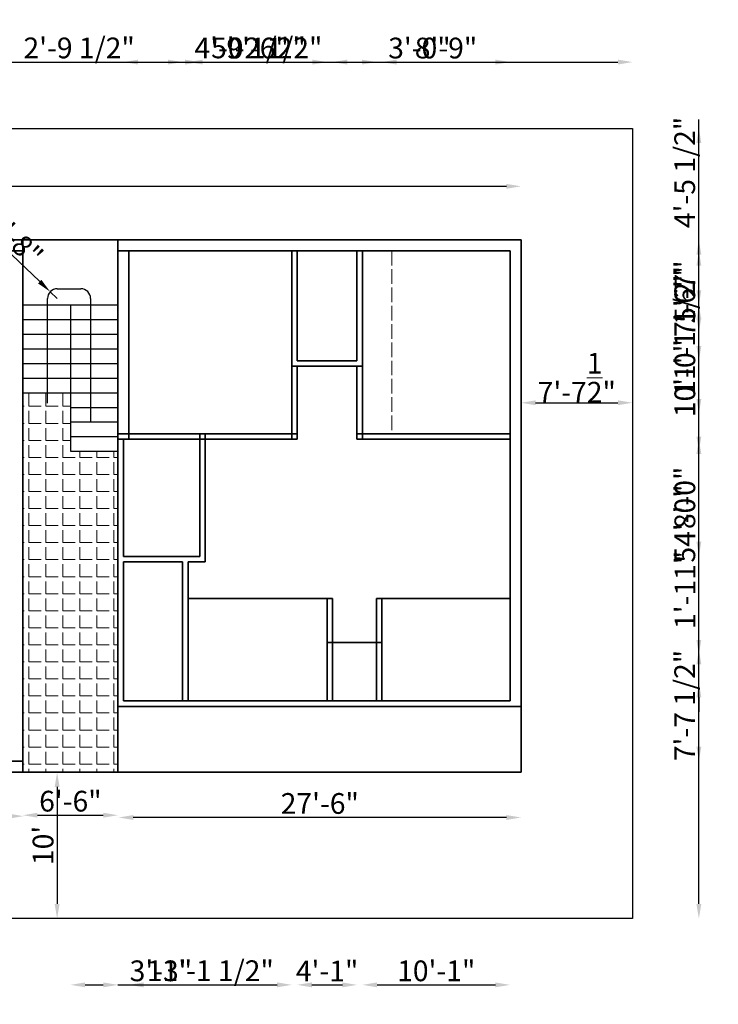
# Model space of a CAD drawing. Units: millimetres. Extents: x 1980 to 3220, y 1535 to 2343.
# Tile 3 of 3: x 2647 to 3220, y 1535 to 2343. Entities that reach past the tile are written whole.
import ezdxf

# ---------------------------------------------------------------- set-up
doc = ezdxf.new("R2010")
doc.units = ezdxf.units.MM
doc.linetypes.add('ACAD_ISO02W100', pattern=[15, 12, -3])
for name, color, linetype, lineweight in [('A-ANNO-DIMS', 2, 'Continuous', 18), ('A-FLOR-FIXT', 9, 'Continuous', 18), ('A-FLOR-FIXT-OVHD', 9, 'ACAD_ISO02W100', 18), ('A-FLOR-PATT', 252, 'Continuous', 13), ('A-FLOR-STRS', 3, 'Continuous', 25), ('A-WALL', 7, 'Continuous', 35), ('C-PROP', 8, 'Continuous', 25)]:
    doc.layers.add(name, color=color, linetype=linetype, lineweight=lineweight)
doc.styles.get("Standard").update_dxf_attribs({"font": 'arial.ttf'})
doc.dimstyles.new('ISO-25', dxfattribs={"dimtxt": 17, "dimasz": 12, "dimexe": 1.25, "dimexo": 0.625, "dimtad": 1, "dimdec": 1, "dimlunit": 4, "dimtxsty": 'Standard', "dimcen": 2.5, "dimse1": 1, "dimse2": 1, "dimadec": 0, "dimazin": 0, "dimtfac": 1, "dimtdec": 1, "dimtmove": 0, "dimatfit": 3, "dimfxl": 1, "dimarcsym": 0})

# ---------------------------------------------------------------- blocks, each defined once
blk = doc.blocks.new('*D1')
at = {"layer": 'A-ANNO-DIMS', "color": 0, "lineweight": -2, "transparency": 16777216}
blk.add_line((2173.01, 2206.08), (3046.01, 2206.08), dxfattribs=at)
at = {"layer": 'A-ANNO-DIMS', "color": 0, "transparency": 16777216}
for points in [[(2173.01, 2208.08), (2173.01, 2204.08), (2161.01, 2206.08)], [(3046.01, 2208.08), (3046.01, 2204.08), (3058.01, 2206.08)]]:
    blk.add_solid(points, dxfattribs=at)
at = {"layer": 'Defpoints', "color": 0, "transparency": 16777216}
for p in [(3058.01, 2206.08), (2161.01, 2162.1), (3058.01, 2162.1)]:
    blk.add_point(p, dxfattribs=at)
at = {"layer": 'A-ANNO-DIMS', "color": 0, "transparency": 16777216, "insert": (2609.51, 2215.39), "char_height": 17, "attachment_point": 5}
blk.add_mtext('74\'-9"', dxfattribs=at)
blk = doc.blocks.new('*D2')
at = {"layer": 'A-ANNO-DIMS', "color": 0, "lineweight": -2, "transparency": 16777216}
blk.add_line((2677.6, 1713.6), (2677.6, 1617.6), dxfattribs=at)
at = {"layer": 'A-ANNO-DIMS', "color": 0, "transparency": 16777216}
for points in [[(2675.6, 1713.6), (2679.6, 1713.6), (2677.6, 1725.6)], [(2675.6, 1617.6), (2679.6, 1617.6), (2677.6, 1605.6)]]:
    blk.add_solid(points, dxfattribs=at)
at = {"layer": 'Defpoints', "color": 0, "transparency": 16777216}
for p in [(2677.6, 1725.6), (2677.6, 1605.6), (2677.6, 1605.6)]:
    blk.add_point(p, dxfattribs=at)
at = {"layer": 'A-ANNO-DIMS', "color": 0, "transparency": 16777216, "insert": (2668.29, 1665.6), "char_height": 17, "attachment_point": 5, "rotation": 90}
blk.add_mtext("10'", dxfattribs=at)
blk = doc.blocks.new('*D3')
at = {"layer": 'A-ANNO-DIMS', "color": 0, "lineweight": -2, "transparency": 16777216}
blk.add_line((2661.51, 1690.37), (2715.51, 1690.37), dxfattribs=at)
at = {"layer": 'A-ANNO-DIMS', "color": 0, "transparency": 16777216}
for points in [[(2661.51, 1692.37), (2661.51, 1688.37), (2649.51, 1690.37)], [(2715.51, 1692.37), (2715.51, 1688.37), (2727.51, 1690.37)]]:
    blk.add_solid(points, dxfattribs=at)
at = {"layer": 'Defpoints', "color": 0, "transparency": 16777216}
for p in [(2649.51, 1725.6), (2727.51, 1725.6), (2727.51, 1690.37)]:
    blk.add_point(p, dxfattribs=at)
at = {"layer": 'A-ANNO-DIMS', "color": 0, "transparency": 16777216, "insert": (2688.51, 1699.68), "char_height": 17, "attachment_point": 5}
blk.add_mtext('6\'-6"', dxfattribs=at)
blk = doc.blocks.new('*D4')
at = {"layer": 'A-ANNO-DIMS', "color": 0, "lineweight": -2, "transparency": 16777216}
blk.add_line((2173.01, 1689.61), (2638.01, 1689.61), dxfattribs=at)
at = {"layer": 'A-ANNO-DIMS', "color": 0, "transparency": 16777216}
for points in [[(2173.01, 1691.61), (2173.01, 1687.61), (2161.01, 1689.61)], [(2638.01, 1691.61), (2638.01, 1687.61), (2650.01, 1689.61)]]:
    blk.add_solid(points, dxfattribs=at)
at = {"layer": 'Defpoints', "color": 0, "transparency": 16777216}
for p in [(2161.01, 1725.6), (2650.01, 1725.6), (2650.01, 1689.61)]:
    blk.add_point(p, dxfattribs=at)
at = {"layer": 'A-ANNO-DIMS', "color": 0, "transparency": 16777216, "insert": (2405.51, 1698.91), "char_height": 17, "attachment_point": 5}
blk.add_mtext('40\'-9"', dxfattribs=at)
blk = doc.blocks.new('*D5')
at = {"layer": 'A-ANNO-DIMS', "color": 0, "lineweight": -2, "transparency": 16777216}
blk.add_line((3046.01, 1688.5), (2740.01, 1688.5), dxfattribs=at)
at = {"layer": 'A-ANNO-DIMS', "color": 0, "transparency": 16777216}
for points in [[(2740.01, 1690.5), (2740.01, 1686.5), (2728.01, 1688.5)], [(3046.01, 1690.5), (3046.01, 1686.5), (3058.01, 1688.5)]]:
    blk.add_solid(points, dxfattribs=at)
at = {"layer": 'Defpoints', "color": 0, "transparency": 16777216}
for p in [(2728.01, 1725.6), (3058.01, 1725.6), (2728.01, 1688.5)]:
    blk.add_point(p, dxfattribs=at)
at = {"layer": 'A-ANNO-DIMS', "color": 0, "transparency": 16777216, "insert": (2893.01, 1697.8), "char_height": 17, "attachment_point": 5}
blk.add_mtext('27\'-6"', dxfattribs=at)
blk = doc.blocks.new('*D6')
at = {"layer": 'A-ANNO-DIMS', "color": 0, "lineweight": -2, "transparency": 16777216}
blk.add_line((3070.01, 2028.59), (3137.51, 2028.59), dxfattribs=at)
at = {"layer": 'A-ANNO-DIMS', "color": 0, "transparency": 16777216}
for points in [[(3070.01, 2030.59), (3070.01, 2026.59), (3058.01, 2028.59)], [(3137.51, 2030.59), (3137.51, 2026.59), (3149.51, 2028.59)]]:
    blk.add_solid(points, dxfattribs=at)
at = {"layer": 'Defpoints', "color": 0, "transparency": 16777216}
for p in [(3149.51, 2028.59), (3058.01, 2011.94), (3149.51, 2011.94)]:
    blk.add_point(p, dxfattribs=at)
at = {"layer": 'A-ANNO-DIMS', "color": 0, "transparency": 16777216, "insert": (3103.76, 2049.12), "char_height": 17, "attachment_point": 5}
blk.add_mtext('7\'-7{\\H1x;\\S1/2;}"', dxfattribs=at)
blk = doc.blocks.new('*D9')
at = {"layer": 'A-ANNO-DIMS', "color": 0, "lineweight": -2, "transparency": 16777216}
blk.add_line((2081.51, 2307.95), (3137.51, 2307.95), dxfattribs=at)
at = {"layer": 'A-ANNO-DIMS', "color": 0, "transparency": 16777216}
for points in [[(2081.51, 2309.95), (2081.51, 2305.95), (2069.51, 2307.95)], [(3137.51, 2309.95), (3137.51, 2305.95), (3149.51, 2307.95)]]:
    blk.add_solid(points, dxfattribs=at)
at = {"layer": 'Defpoints', "color": 0, "transparency": 16777216}
for p in [(3149.51, 2307.95), (2069.51, 2253.6), (3149.51, 2253.6)]:
    blk.add_point(p, dxfattribs=at)
at = {"layer": 'A-ANNO-DIMS', "color": 0, "transparency": 16777216, "insert": (2609.51, 2317.25), "char_height": 17, "attachment_point": 5}
blk.add_mtext('90\'-0"', dxfattribs=at)
blk = doc.blocks.new('*D10')
at = {"layer": 'A-ANNO-DIMS', "color": 0, "lineweight": -2, "transparency": 16777216}
blk.add_line((3203.86, 1617.6), (3203.86, 2241.6), dxfattribs=at)
at = {"layer": 'A-ANNO-DIMS', "color": 0, "transparency": 16777216}
for points in [[(3201.86, 2241.6), (3205.86, 2241.6), (3203.86, 2253.6)], [(3201.86, 1617.6), (3205.86, 1617.6), (3203.86, 1605.6)]]:
    blk.add_solid(points, dxfattribs=at)
at = {"layer": 'Defpoints', "color": 0, "transparency": 16777216}
for p in [(3149.51, 2253.6), (3203.86, 2253.6), (3149.51, 1605.6)]:
    blk.add_point(p, dxfattribs=at)
at = {"layer": 'A-ANNO-DIMS', "color": 0, "transparency": 16777216, "insert": (3194.55, 1929.6), "char_height": 17, "attachment_point": 5, "rotation": 90}
blk.add_mtext('54\'-0"', dxfattribs=at)
blk = doc.blocks.new('*D15')
at = {"layer": 'A-ANNO-DIMS', "color": 0, "lineweight": -2, "transparency": 16777216}
blk.add_line((3203.86, 2031.6), (3203.86, 2141.1), dxfattribs=at)
at = {"layer": 'A-ANNO-DIMS', "color": 0, "transparency": 16777216}
for points in [[(3201.86, 2141.1), (3205.86, 2141.1), (3203.86, 2153.1)], [(3201.86, 2031.6), (3205.86, 2031.6), (3203.86, 2019.6)]]:
    blk.add_solid(points, dxfattribs=at)
at = {"layer": 'Defpoints', "color": 0, "transparency": 16777216}
for p in [(2170.01, 2153.1), (3203.86, 2153.1), (2170.01, 2019.6)]:
    blk.add_point(p, dxfattribs=at)
at = {"layer": 'A-ANNO-DIMS', "color": 0, "transparency": 16777216, "insert": (3194.44, 2086.35), "char_height": 17, "attachment_point": 5, "rotation": 90}
blk.add_mtext('11\'-1 1/2"', dxfattribs=at)
blk = doc.blocks.new('*D16')
at = {"layer": 'A-ANNO-DIMS', "color": 0, "lineweight": -2, "transparency": 16777216}
blk.add_line((3203.86, 2075.1), (3203.86, 2141.1), dxfattribs=at)
at = {"layer": 'A-ANNO-DIMS', "color": 0, "transparency": 16777216}
for points in [[(3201.86, 2141.1), (3205.86, 2141.1), (3203.86, 2153.1)], [(3201.86, 2075.1), (3205.86, 2075.1), (3203.86, 2063.1)]]:
    blk.add_solid(points, dxfattribs=at)
at = {"layer": 'Defpoints', "color": 0, "transparency": 16777216}
for p in [(2357.51, 2153.1), (3203.86, 2153.1), (2357.51, 2063.1)]:
    blk.add_point(p, dxfattribs=at)
at = {"layer": 'A-ANNO-DIMS', "color": 0, "transparency": 16777216, "insert": (3194.55, 2108.1), "char_height": 17, "attachment_point": 5, "rotation": 90}
blk.add_mtext('7\'-6"', dxfattribs=at)
blk = doc.blocks.new('*D27')
at = {"layer": 'A-ANNO-DIMS', "color": 0, "lineweight": -2, "transparency": 16777216}
blk.add_line((3203.86, 1746.6), (3203.86, 1814.1), dxfattribs=at)
at = {"layer": 'A-ANNO-DIMS', "color": 0, "transparency": 16777216}
for points in [[(3201.86, 1814.1), (3205.86, 1814.1), (3203.86, 1826.1)], [(3201.86, 1746.6), (3205.86, 1746.6), (3203.86, 1734.6)]]:
    blk.add_solid(points, dxfattribs=at)
at = {"layer": 'Defpoints', "color": 0, "transparency": 16777216}
for p in [(2278.01, 1826.1), (3203.86, 1826.1), (2278.01, 1734.6)]:
    blk.add_point(p, dxfattribs=at)
at = {"layer": 'A-ANNO-DIMS', "color": 0, "transparency": 16777216, "insert": (3194.44, 1780.35), "char_height": 17, "attachment_point": 5, "rotation": 90}
blk.add_mtext('7\'-7 1/2"', dxfattribs=at)
blk = doc.blocks.new('*D30')
at = {"layer": 'A-ANNO-DIMS', "color": 0, "lineweight": -2, "transparency": 16777216}
for p, q in [((2619.26, 2307.95), (2628.51, 2307.95)), ((2640.51, 2307.95), (2738.85, 2307.95))]:
    blk.add_line(p, q, dxfattribs=at)
at = {"layer": 'A-ANNO-DIMS', "color": 0, "transparency": 16777216}
for points in [[(2619.26, 2309.95), (2619.26, 2305.95), (2607.26, 2307.95)], [(2628.51, 2309.95), (2628.51, 2305.95), (2640.51, 2307.95)]]:
    blk.add_solid(points, dxfattribs=at)
at = {"layer": 'Defpoints', "color": 0, "transparency": 16777216}
for p in [(2640.51, 2307.95), (2607.26, 1734.6), (2640.51, 1734.6)]:
    blk.add_point(p, dxfattribs=at)
at = {"layer": 'A-ANNO-DIMS', "color": 0, "transparency": 16777216, "insert": (2695.68, 2317.36), "char_height": 17, "attachment_point": 5}
blk.add_mtext('2\'-9 1/2"', dxfattribs=at)
blk = doc.blocks.new('*D31')
at = {"layer": 'A-ANNO-DIMS', "color": 0, "lineweight": -2, "transparency": 16777216}
blk.add_line((2748.51, 1551.25), (2858.01, 1551.25), dxfattribs=at)
at = {"layer": 'A-ANNO-DIMS', "color": 0, "transparency": 16777216}
for points in [[(2748.51, 1553.25), (2748.51, 1549.25), (2736.51, 1551.25)], [(2858.01, 1553.25), (2858.01, 1549.25), (2870.01, 1551.25)]]:
    blk.add_solid(points, dxfattribs=at)
at = {"layer": 'Defpoints', "color": 0, "transparency": 16777216}
for p in [(2736.51, 2153.1), (2870.01, 2153.1), (2870.01, 1551.25)]:
    blk.add_point(p, dxfattribs=at)
at = {"layer": 'A-ANNO-DIMS', "color": 0, "transparency": 16777216, "insert": (2803.26, 1560.66), "char_height": 17, "attachment_point": 5}
blk.add_mtext('11\'-1 1/2"', dxfattribs=at)
blk = doc.blocks.new('*D32')
at = {"layer": 'A-ANNO-DIMS', "color": 0, "lineweight": -2, "transparency": 16777216}
blk.add_line((2886.51, 1551.25), (2911.51, 1551.25), dxfattribs=at)
at = {"layer": 'A-ANNO-DIMS', "color": 0, "transparency": 16777216}
for points in [[(2886.51, 1553.25), (2886.51, 1549.25), (2874.51, 1551.25)], [(2911.51, 1553.25), (2911.51, 1549.25), (2923.51, 1551.25)]]:
    blk.add_solid(points, dxfattribs=at)
at = {"layer": 'Defpoints', "color": 0, "transparency": 16777216}
for p in [(2874.51, 2153.1), (2923.51, 2153.1), (2923.51, 1551.25)]:
    blk.add_point(p, dxfattribs=at)
at = {"layer": 'A-ANNO-DIMS', "color": 0, "transparency": 16777216, "insert": (2899.01, 1560.41), "char_height": 17, "attachment_point": 5}
blk.add_mtext('4\'-1"', dxfattribs=at)
blk = doc.blocks.new('*D33')
at = {"layer": 'A-ANNO-DIMS', "color": 0, "lineweight": -2, "transparency": 16777216}
blk.add_line((2940.01, 1551.25), (3037.01, 1551.25), dxfattribs=at)
at = {"layer": 'A-ANNO-DIMS', "color": 0, "transparency": 16777216}
for points in [[(2940.01, 1553.25), (2940.01, 1549.25), (2928.01, 1551.25)], [(3037.01, 1553.25), (3037.01, 1549.25), (3049.01, 1551.25)]]:
    blk.add_solid(points, dxfattribs=at)
at = {"layer": 'Defpoints', "color": 0, "transparency": 16777216}
for p in [(2928.01, 2153.1), (3049.01, 2153.1), (3049.01, 1551.25)]:
    blk.add_point(p, dxfattribs=at)
at = {"layer": 'A-ANNO-DIMS', "color": 0, "transparency": 16777216, "insert": (2988.51, 1560.55), "char_height": 17, "attachment_point": 5}
blk.add_mtext('10\'-1"', dxfattribs=at)
blk = doc.blocks.new('*D34')
at = {"layer": 'A-ANNO-DIMS', "color": 0, "lineweight": -2, "transparency": 16777216}
blk.add_line((2015.16, 2015.1), (2015.16, 2141.1), dxfattribs=at)
at = {"layer": 'A-ANNO-DIMS', "color": 0, "transparency": 16777216}
for points in [[(2013.16, 2141.1), (2017.16, 2141.1), (2015.16, 2153.1)], [(2013.16, 2015.1), (2017.16, 2015.1), (2015.16, 2003.1)]]:
    blk.add_solid(points, dxfattribs=at)
at = {"layer": 'Defpoints', "color": 0, "transparency": 16777216}
for p in [(2015.16, 2153.1), (3049.01, 2153.1), (3049.01, 2003.1)]:
    blk.add_point(p, dxfattribs=at)
at = {"layer": 'A-ANNO-DIMS', "color": 0, "transparency": 16777216, "insert": (2005.85, 2078.1), "char_height": 17, "attachment_point": 5, "rotation": 90}
blk.add_mtext('12\'-6"', dxfattribs=at)
blk = doc.blocks.new('*D35')
at = {"layer": 'A-ANNO-DIMS', "color": 0, "lineweight": -2, "transparency": 16777216}
blk.add_line((2015.16, 2075.1), (2015.16, 2141.1), dxfattribs=at)
at = {"layer": 'A-ANNO-DIMS', "color": 0, "transparency": 16777216}
for points in [[(2013.16, 2141.1), (2017.16, 2141.1), (2015.16, 2153.1)], [(2013.16, 2075.1), (2017.16, 2075.1), (2015.16, 2063.1)]]:
    blk.add_solid(points, dxfattribs=at)
at = {"layer": 'Defpoints', "color": 0, "transparency": 16777216}
for p in [(2015.16, 2153.1), (2923.51, 2153.1), (2923.51, 2063.1)]:
    blk.add_point(p, dxfattribs=at)
at = {"layer": 'A-ANNO-DIMS', "color": 0, "transparency": 16777216, "insert": (2005.85, 2108.1), "char_height": 17, "attachment_point": 5, "rotation": 90}
blk.add_mtext('7\'-6"', dxfattribs=at)
blk = doc.blocks.new('*D36')
at = {"layer": 'A-ANNO-DIMS', "color": 0, "lineweight": -2, "transparency": 16777216}
for p, q in [((2744.01, 2307.95), (2782.51, 2307.95)), ((2794.51, 2307.95), (2892.56, 2307.95))]:
    blk.add_line(p, q, dxfattribs=at)
at = {"layer": 'A-ANNO-DIMS', "color": 0, "transparency": 16777216}
for points in [[(2744.01, 2309.95), (2744.01, 2305.95), (2732.01, 2307.95)], [(2782.51, 2309.95), (2782.51, 2305.95), (2794.51, 2307.95)]]:
    blk.add_solid(points, dxfattribs=at)
at = {"layer": 'Defpoints', "color": 0, "transparency": 16777216}
for p in [(2794.51, 2307.95), (2732.01, 1902.6), (2794.51, 1902.6)]:
    blk.add_point(p, dxfattribs=at)
at = {"layer": 'A-ANNO-DIMS', "color": 0, "transparency": 16777216, "insert": (2849.53, 2317.36), "char_height": 17, "attachment_point": 5}
blk.add_mtext('5\'-2 1/2"', dxfattribs=at)
blk = doc.blocks.new('*D37')
at = {"layer": 'A-ANNO-DIMS', "color": 0, "lineweight": -2, "transparency": 16777216}
blk.add_line((3203.86, 1914.6), (3203.86, 1986.6), dxfattribs=at)
at = {"layer": 'A-ANNO-DIMS', "color": 0, "transparency": 16777216}
for points in [[(3201.86, 1986.6), (3205.86, 1986.6), (3203.86, 1998.6)], [(3201.86, 1914.6), (3205.86, 1914.6), (3203.86, 1902.6)]]:
    blk.add_solid(points, dxfattribs=at)
at = {"layer": 'Defpoints', "color": 0, "transparency": 16777216}
for p in [(2732.01, 1998.6), (3203.86, 1998.6), (2732.01, 1902.6)]:
    blk.add_point(p, dxfattribs=at)
at = {"layer": 'A-ANNO-DIMS', "color": 0, "transparency": 16777216, "insert": (3194.55, 1950.6), "char_height": 17, "attachment_point": 5, "rotation": 90}
blk.add_mtext('8\'-0"', dxfattribs=at)
blk = doc.blocks.new('*D38')
at = {"layer": 'A-ANNO-DIMS', "color": 0, "lineweight": -2, "transparency": 16777216}
for p, q in [((2744.01, 2307.95), (2768.51, 2307.95)), ((2780.51, 2307.95), (2879.25, 2307.95))]:
    blk.add_line(p, q, dxfattribs=at)
at = {"layer": 'A-ANNO-DIMS', "color": 0, "transparency": 16777216}
for points in [[(2744.01, 2309.95), (2744.01, 2305.95), (2732.01, 2307.95)], [(2768.51, 2309.95), (2768.51, 2305.95), (2780.51, 2307.95)]]:
    blk.add_solid(points, dxfattribs=at)
at = {"layer": 'Defpoints', "color": 0, "transparency": 16777216}
for p in [(2780.51, 2307.95), (2732.01, 1784.1), (2780.51, 1784.1)]:
    blk.add_point(p, dxfattribs=at)
at = {"layer": 'A-ANNO-DIMS', "color": 0, "transparency": 16777216, "insert": (2835.88, 2317.36), "char_height": 17, "attachment_point": 5}
blk.add_mtext('4\'-0 1/2"', dxfattribs=at)
blk = doc.blocks.new('*D39')
at = {"layer": 'A-ANNO-DIMS', "color": 0, "lineweight": -2, "transparency": 16777216}
blk.add_line((2797.01, 2307.95), (2887.01, 2307.95), dxfattribs=at)
at = {"layer": 'A-ANNO-DIMS', "color": 0, "transparency": 16777216}
for points in [[(2797.01, 2309.95), (2797.01, 2305.95), (2785.01, 2307.95)], [(2887.01, 2309.95), (2887.01, 2305.95), (2899.01, 2307.95)]]:
    blk.add_solid(points, dxfattribs=at)
at = {"layer": 'Defpoints', "color": 0, "transparency": 16777216}
for p in [(2899.01, 2307.95), (2785.01, 1784.1), (2899.01, 1784.1)]:
    blk.add_point(p, dxfattribs=at)
at = {"layer": 'A-ANNO-DIMS', "color": 0, "transparency": 16777216, "insert": (2842.01, 2317.25), "char_height": 17, "attachment_point": 5}
blk.add_mtext('9\'-6"', dxfattribs=at)
blk = doc.blocks.new('*D40')
at = {"layer": 'A-ANNO-DIMS', "color": 0, "lineweight": -2, "transparency": 16777216}
for p, q in [((2915.51, 2307.95), (2927.51, 2307.95)), ((2939.51, 2307.95), (2997.94, 2307.95))]:
    blk.add_line(p, q, dxfattribs=at)
at = {"layer": 'A-ANNO-DIMS', "color": 0, "transparency": 16777216}
for points in [[(2915.51, 2309.95), (2915.51, 2305.95), (2903.51, 2307.95)], [(2927.51, 2309.95), (2927.51, 2305.95), (2939.51, 2307.95)]]:
    blk.add_solid(points, dxfattribs=at)
at = {"layer": 'Defpoints', "color": 0, "transparency": 16777216}
for p in [(2939.51, 2307.95), (2903.51, 1784.1), (2939.51, 1784.1)]:
    blk.add_point(p, dxfattribs=at)
at = {"layer": 'A-ANNO-DIMS', "color": 0, "transparency": 16777216, "insert": (2974.72, 2317.26), "char_height": 17, "attachment_point": 5}
blk.add_mtext('3\'-0"', dxfattribs=at)
blk = doc.blocks.new('*D41')
at = {"layer": 'A-ANNO-DIMS', "color": 0, "lineweight": -2, "transparency": 16777216}
blk.add_line((2956.01, 2307.95), (3037.01, 2307.95), dxfattribs=at)
at = {"layer": 'A-ANNO-DIMS', "color": 0, "transparency": 16777216}
for points in [[(2956.01, 2309.95), (2956.01, 2305.95), (2944.01, 2307.95)], [(3037.01, 2309.95), (3037.01, 2305.95), (3049.01, 2307.95)]]:
    blk.add_solid(points, dxfattribs=at)
at = {"layer": 'Defpoints', "color": 0, "transparency": 16777216}
for p in [(3049.01, 2307.95), (2944.01, 1784.1), (3049.01, 1784.1)]:
    blk.add_point(p, dxfattribs=at)
at = {"layer": 'A-ANNO-DIMS', "color": 0, "transparency": 16777216, "insert": (2996.51, 2317.25), "char_height": 17, "attachment_point": 5}
blk.add_mtext('8\'-9"', dxfattribs=at)
blk = doc.blocks.new('*D42')
at = {"layer": 'A-ANNO-DIMS', "color": 0, "lineweight": -2, "transparency": 16777216}
blk.add_line((2015.16, 1796.1), (2015.16, 1856.1), dxfattribs=at)
at = {"layer": 'A-ANNO-DIMS', "color": 0, "transparency": 16777216}
for points in [[(2013.16, 1856.1), (2017.16, 1856.1), (2015.16, 1868.1)], [(2013.16, 1796.1), (2017.16, 1796.1), (2015.16, 1784.1)]]:
    blk.add_solid(points, dxfattribs=at)
at = {"layer": 'Defpoints', "color": 0, "transparency": 16777216}
for p in [(2015.16, 1868.1), (3049.01, 1868.1), (3049.01, 1784.1)]:
    blk.add_point(p, dxfattribs=at)
at = {"layer": 'A-ANNO-DIMS', "color": 0, "transparency": 16777216, "insert": (2005.85, 1826.1), "char_height": 17, "attachment_point": 5, "rotation": 90}
blk.add_mtext('7\'-0"', dxfattribs=at)
blk = doc.blocks.new('*D43')
at = {"layer": 'A-ANNO-DIMS', "color": 0, "lineweight": -2, "transparency": 16777216}
blk.add_line((2015.16, 1796.1), (2015.16, 1820.1), dxfattribs=at)
at = {"layer": 'A-ANNO-DIMS', "color": 0, "transparency": 16777216}
for points in [[(2013.16, 1820.1), (2017.16, 1820.1), (2015.16, 1832.1)], [(2013.16, 1796.1), (2017.16, 1796.1), (2015.16, 1784.1)]]:
    blk.add_solid(points, dxfattribs=at)
at = {"layer": 'Defpoints', "color": 0, "transparency": 16777216}
for p in [(2015.16, 1832.1), (2944.01, 1832.1), (2939.51, 1784.1)]:
    blk.add_point(p, dxfattribs=at)
at = {"layer": 'A-ANNO-DIMS', "color": 0, "transparency": 16777216, "insert": (2005.85, 1808.1), "char_height": 17, "attachment_point": 5, "rotation": 90}
blk.add_mtext('4\'-0"', dxfattribs=at)
blk = doc.blocks.new('*D44')
at = {"layer": 'A-ANNO-DIMS', "color": 0, "lineweight": -2, "transparency": 16777216}
blk.add_line((2015.16, 1737.6), (2015.16, 1767.6), dxfattribs=at)
at = {"layer": 'A-ANNO-DIMS', "color": 0, "transparency": 16777216}
for points in [[(2013.16, 1767.6), (2017.16, 1767.6), (2015.16, 1779.6)], [(2013.16, 1737.6), (2017.16, 1737.6), (2015.16, 1725.6)]]:
    blk.add_solid(points, dxfattribs=at)
at = {"layer": 'Defpoints', "color": 0, "transparency": 16777216}
for p in [(2015.16, 1779.6), (3058.01, 1779.6), (3058.01, 1725.6)]:
    blk.add_point(p, dxfattribs=at)
at = {"layer": 'A-ANNO-DIMS', "color": 0, "transparency": 16777216, "insert": (2005.85, 1752.6), "char_height": 17, "attachment_point": 5, "rotation": 90}
blk.add_mtext('4\'-6"', dxfattribs=at)
blk = doc.blocks.new('*D45')
at = {"layer": 'A-ANNO-DIMS', "color": 0, "lineweight": -2, "transparency": 16777216}
blk.add_line((3203.86, 2000.82), (3203.86, 2096.82), dxfattribs=at)
at = {"layer": 'A-ANNO-DIMS', "color": 0, "transparency": 16777216}
for points in [[(3201.86, 2096.82), (3205.86, 2096.82), (3203.86, 2108.82)], [(3201.86, 2000.82), (3205.86, 2000.82), (3203.86, 1988.82)]]:
    blk.add_solid(points, dxfattribs=at)
at = {"layer": 'Defpoints', "color": 0, "transparency": 16777216}
for p in [(2727.51, 2108.82), (3203.86, 2108.82), (2727.51, 1988.82)]:
    blk.add_point(p, dxfattribs=at)
at = {"layer": 'A-ANNO-DIMS', "color": 0, "transparency": 16777216, "insert": (3194.55, 2048.82), "char_height": 17, "attachment_point": 5, "rotation": 90}
blk.add_mtext('10\'-0"', dxfattribs=at)
blk = doc.blocks.new('*D46')
at = {"layer": 'A-ANNO-DIMS', "color": 0, "lineweight": -2, "transparency": 16777216}
for p, q in [((3203.86, 2162.1), (3203.86, 2260.83)), ((3203.86, 2120.82), (3203.86, 2150.1))]:
    blk.add_line(p, q, dxfattribs=at)
at = {"layer": 'A-ANNO-DIMS', "color": 0, "transparency": 16777216}
for points in [[(3201.86, 2150.1), (3205.86, 2150.1), (3203.86, 2162.1)], [(3201.86, 2120.82), (3205.86, 2120.82), (3203.86, 2108.82)]]:
    blk.add_solid(points, dxfattribs=at)
at = {"layer": 'Defpoints', "color": 0, "transparency": 16777216}
for p in [(2727.51, 2162.1), (3203.86, 2162.1), (2727.51, 2108.82)]:
    blk.add_point(p, dxfattribs=at)
at = {"layer": 'A-ANNO-DIMS', "color": 0, "transparency": 16777216, "insert": (3194.44, 2217.46), "char_height": 17, "attachment_point": 5, "rotation": 90}
blk.add_mtext('4\'-5 1/2"', dxfattribs=at)
blk = doc.blocks.new('*D47')
at = {"layer": 'A-ANNO-DIMS', "color": 0, "lineweight": -2, "transparency": 16777216}
for p, q in [((2700.51, 1551.25), (2715.51, 1551.25)), ((2727.51, 1551.25), (2785.94, 1551.25))]:
    blk.add_line(p, q, dxfattribs=at)
at = {"layer": 'A-ANNO-DIMS', "color": 0, "transparency": 16777216}
for points in [[(2700.51, 1553.25), (2700.51, 1549.25), (2688.51, 1551.25)], [(2715.51, 1553.25), (2715.51, 1549.25), (2727.51, 1551.25)]]:
    blk.add_solid(points, dxfattribs=at)
at = {"layer": 'Defpoints', "color": 0, "transparency": 16777216}
for p in [(2688.51, 1988.82), (2727.51, 1988.82), (2727.51, 1551.25)]:
    blk.add_point(p, dxfattribs=at)
at = {"layer": 'A-ANNO-DIMS', "color": 0, "transparency": 16777216, "insert": (2762.72, 1560.56), "char_height": 17, "attachment_point": 5}
blk.add_mtext('3\'-3"', dxfattribs=at)
blk = doc.blocks.new('*D48')
at = {"layer": 'A-ANNO-DIMS', "color": 0, "lineweight": -2, "transparency": 16777216}
for p, q in [((2015.16, 2120.82), (2015.16, 2177.66)), ((2015.16, 2096.82), (2015.16, 2108.82)), ((2015.16, 2084.82), (2015.16, 2072.82))]:
    blk.add_line(p, q, dxfattribs=at)
at = {"layer": 'A-ANNO-DIMS', "color": 0, "transparency": 16777216}
for points in [[(2013.16, 2120.82), (2017.16, 2120.82), (2015.16, 2108.82)], [(2013.16, 2084.82), (2017.16, 2084.82), (2015.16, 2096.82)]]:
    blk.add_solid(points, dxfattribs=at)
at = {"layer": 'Defpoints', "color": 0, "transparency": 16777216}
for p in [(2015.16, 2108.82), (2649.51, 2108.82), (2649.51, 2096.82)]:
    blk.add_point(p, dxfattribs=at)
at = {"layer": 'A-ANNO-DIMS', "color": 0, "transparency": 16777216, "insert": (2005.85, 2155.24), "char_height": 17, "attachment_point": 5, "rotation": 90}
blk.add_mtext('1\'-0"', dxfattribs=at)
blk = doc.blocks.new('*D52')
at = {"layer": 'A-ANNO-DIMS', "color": 0, "lineweight": -2, "transparency": 16777216}
blk.add_line((3203.86, 2098.35), (3203.86, 2141.1), dxfattribs=at)
at = {"layer": 'A-ANNO-DIMS', "color": 0, "transparency": 16777216}
for points in [[(3201.86, 2141.1), (3205.86, 2141.1), (3203.86, 2153.1)], [(3201.86, 2098.35), (3205.86, 2098.35), (3203.86, 2086.35)]]:
    blk.add_solid(points, dxfattribs=at)
at = {"layer": 'Defpoints', "color": 0, "transparency": 16777216}
for p in [(2538.69, 2153.1), (3203.86, 2153.1), (2510.51, 2086.35)]:
    blk.add_point(p, dxfattribs=at)
at = {"layer": 'A-ANNO-DIMS', "color": 0, "transparency": 16777216, "insert": (3194.59, 2119.72), "char_height": 17, "attachment_point": 5, "rotation": 90}
blk.add_mtext('5\'-7"', dxfattribs=at)
blk = doc.blocks.new('*D55')
at = {"layer": 'A-ANNO-DIMS', "color": 0, "lineweight": -2, "transparency": 16777216}
for p, q in [((3203.86, 1834.1), (3203.86, 1904.15)), ((3203.86, 1799.1), (3203.86, 1822.1)), ((3203.86, 1787.1), (3203.86, 1775.1))]:
    blk.add_line(p, q, dxfattribs=at)
at = {"layer": 'A-ANNO-DIMS', "color": 0, "transparency": 16777216}
for points in [[(3201.86, 1834.1), (3205.86, 1834.1), (3203.86, 1822.1)], [(3201.86, 1787.1), (3205.86, 1787.1), (3203.86, 1799.1)]]:
    blk.add_solid(points, dxfattribs=at)
at = {"layer": 'Defpoints', "color": 0, "transparency": 16777216}
for p in [(2482.01, 1822.1), (3203.86, 1822.1), (2482.01, 1799.1)]:
    blk.add_point(p, dxfattribs=at)
at = {"layer": 'A-ANNO-DIMS', "color": 0, "transparency": 16777216, "insert": (3194.7, 1875.12), "char_height": 17, "attachment_point": 5, "rotation": 90}
blk.add_mtext('1\'-11"', dxfattribs=at)
blk = doc.blocks.new('*D58')
at = {"layer": 'A-ANNO-DIMS', "color": 0, "lineweight": -2, "transparency": 16777216}
for p, q in [((2582.78, 2205.03), (2663.33, 2127.9)), ((2677.78, 2114.07), (2672, 2119.6))]:
    blk.add_line(p, q, dxfattribs=at)
at = {"layer": 'A-ANNO-DIMS', "color": 0, "transparency": 16777216}
blk.add_solid([(2664.72, 2129.34), (2661.95, 2126.45), (2672, 2119.6)], dxfattribs=at)
at = {"layer": 'Defpoints', "color": 0, "transparency": 16777216}
for p in [(2672, 2119.6), (2677.78, 2114.07)]:
    blk.add_point(p, dxfattribs=at)
at = {"layer": 'A-ANNO-DIMS', "color": 0, "transparency": 16777216, "insert": (2625.16, 2177.34), "char_height": 17, "attachment_point": 5, "rotation": 316.24382}
blk.add_mtext('2X R0\'-8"', dxfattribs=at)

msp = doc.modelspace()

# ---------------------------------------------------------------- hatches: boundary and pattern name
at = {"layer": 'A-FLOR-PATT'}
h = msp.add_hatch(dxfattribs=at)
h.set_pattern_fill('ANGLE', color=256, scale=2)
h.set_pattern_definition([(0, (0, 0), (0, 13.97), [10.16, -3.81]), (90, (0, 0), (-13.97, 9e-16), [10.16, -3.81])])
h.paths.add_polyline_path([(2727.51, 1988.82), (2688.51, 1988.82), (2688.51, 2036.82), (2649.51, 2036.82), (2649.51, 1725.6), (2727.51, 1725.6)])
h.paths.add_polyline_path([(2273.51, 1826.1), (2165.51, 1826.1), (2165.51, 1734.6), (2273.51, 1734.6)])

# ---------------------------------------------------------------- linework, layer by layer
at = {"layer": 'A-FLOR-FIXT'}
msp.add_line((2928.01, 2153.1), (2952.01, 2153.1), dxfattribs=at)
at = {"layer": 'A-FLOR-FIXT-OVHD'}
msp.add_line((2952.01, 2153.1), (2952.01, 2003.1), dxfattribs=at)
at = {"layer": 'A-FLOR-STRS'}
for p, q in [((2677.78, 2122.07), (2697.08, 2122.07)), ((2649.51, 2108.82), (2727.51, 2108.82)), ((2669.78, 2028.31), (2669.78, 2114.07)), ((2688.51, 2108.82), (2688.51, 2036.82)), ((2705.08, 2114.07), (2705.08, 2012.82)), ((2649.51, 2096.82), (2727.51, 2096.82)), ((2649.51, 2084.82), (2727.51, 2084.82)), ((2649.51, 2072.82), (2727.51, 2072.82)), ((2649.51, 2060.82), (2727.51, 2060.82)), ((2649.51, 2048.82), (2727.51, 2048.82)), ((2649.51, 2036.82), (2688.51, 2036.82)), ((2688.51, 2036.82), (2727.51, 2036.82)), ((2688.51, 2036.82), (2688.51, 1988.82)), ((2688.51, 2024.82), (2727.51, 2024.82)), ((2688.51, 2012.82), (2727.51, 2012.82)), ((2688.51, 2000.82), (2727.51, 2000.82)), ((2688.51, 1988.82), (2727.51, 1988.82))]:
    msp.add_line(p, q, dxfattribs=at)
for centre, start, end in [((2677.78, 2114.07), 90, 180), ((2697.08, 2114.07), 0, 90)]:
    msp.add_arc(centre, 8, start, end, dxfattribs=at)
at = {"layer": 'A-WALL'}
for p, q in [((2161.01, 2162.1), (3058.01, 2162.1)), ((2649.51, 1725.6), (2649.51, 2162.1)), ((2727.51, 1725.6), (2727.51, 2162.1)), ((3058.01, 2162.1), (3058.01, 1725.6)), ((2170.01, 2153.1), (2649.51, 2153.1)), ((2727.51, 2153.1), (3049.01, 2153.1)), ((2736.51, 1998.6), (2736.51, 2153.1)), ((2870.01, 1998.6), (2870.01, 2153.1)), ((2874.51, 2063.1), (2874.51, 2153.1)), ((2923.51, 2063.1), (2923.51, 2153.1)), ((2928.01, 1998.6), (2928.01, 2153.1)), ((3049.01, 2153.1), (3049.01, 1784.1)), ((2874.51, 2063.1), (2923.51, 2063.1)), ((2870.01, 2058.6), (2928.01, 2058.6)), ((2874.51, 1998.6), (2874.51, 2058.6)), ((2923.51, 1998.6), (2923.51, 2058.6)), ((2727.51, 2003.1), (2874.51, 2003.1)), ((2794.51, 1902.6), (2794.51, 2003.1)), ((2799.01, 1898.1), (2799.01, 2003.1)), ((2923.51, 2003.1), (3049.01, 2003.1)), ((2727.51, 1998.6), (2874.51, 1998.6)), ((2732.01, 1902.6), (2732.01, 1998.6)), ((2923.51, 1998.6), (3049.01, 1998.6)), ((2732.01, 1902.6), (2794.51, 1902.6)), ((2732.01, 1898.1), (2780.51, 1898.1)), ((2732.01, 1784.1), (2732.01, 1898.1)), ((2780.51, 1898.1), (2780.51, 1784.1)), ((2785.01, 1898.1), (2785.01, 1784.1)), ((2785.01, 1898.1), (2799.01, 1898.1)), ((2903.51, 1868.1), (2785.01, 1868.1)), ((2899.01, 1868.1), (2899.01, 1784.1)), ((2903.51, 1868.1), (2903.51, 1784.1)), ((3049.01, 1868.1), (2939.51, 1868.1)), ((2939.51, 1868.1), (2939.51, 1784.1)), ((2944.01, 1868.1), (2944.01, 1784.1)), ((2944.01, 1832.1), (2899.01, 1832.1)), ((2727.51, 1779.6), (3058.01, 1779.6)), ((2732.01, 1784.1), (3049.01, 1784.1)), ((2649.51, 1734.6), (2607.26, 1734.6)), ((3058.01, 1725.6), (2161.01, 1725.6)), ((2727.51, 1725.6), (3058.01, 1725.6))]:
    msp.add_line(p, q, dxfattribs=at)
at = {"layer": 'C-PROP'}
msp.add_lwpolyline([(2069.51, 2253.6), (3149.51, 2253.6), (3149.51, 1605.6), (2069.51, 1605.6)], close=True, dxfattribs=at)

# ---------------------------------------------------------------- dimensions: what is measured, and where the dimension line sits
at = {"layer": 'A-ANNO-DIMS'}
for base, p1, p2, override, picture, middle in [((2640.508481, 2307.945639), (2607.258481, 1734.595639), (2640.508481, 1734.595639), {"dimdec": 1, "dimlfac": 1, "dimrnd": 0, "dimzin": 1, "dimdsep": 46, "dimlunit": 4, "dimfrac": 2}, '*D30', (2695.67986572, 2317.3605435)), ((2794.51, 2307.95), (2732.01, 1902.6), (2794.51, 1902.6), {"dimdec": 1, "dimlfac": 1, "dimrnd": 0, "dimzin": 1, "dimdsep": 46, "dimlunit": 4, "dimfrac": 2}, '*D36', (2849.53, 2317.36)), ((2780.51, 2307.95), (2732.01, 1784.1), (2780.51, 1784.1), {"dimdec": 1, "dimlfac": 1, "dimrnd": 0, "dimzin": 1, "dimdsep": 46, "dimlunit": 4, "dimfrac": 2}, '*D38', (2835.88, 2317.36)), ((3149.51, 2307.95), (2069.51, 2253.6), (3149.51, 2253.6), {"dimdec": 1, "dimlfac": 1, "dimrnd": 0, "dimzin": 1, "dimdsep": 46, "dimlunit": 4, "dimfrac": 2}, '*D9', (2609.51, 2317.25)), ((2899.01, 2307.95), (2785.01, 1784.1), (2899.01, 1784.1), {"dimdec": 1, "dimlfac": 1, "dimrnd": 0, "dimzin": 1, "dimdsep": 46, "dimlunit": 4, "dimfrac": 2}, '*D39', (2842.01, 2317.25)), ((2939.51, 2307.95), (2903.51, 1784.1), (2939.51, 1784.1), {"dimdec": 1, "dimlfac": 1, "dimrnd": 0, "dimzin": 1, "dimdsep": 46, "dimlunit": 4, "dimfrac": 2}, '*D40', (2974.72, 2317.26)), ((3049.01, 2307.95), (2944.01, 1784.1), (3049.01, 1784.1), {"dimdec": 1, "dimlfac": 1, "dimrnd": 0, "dimzin": 1, "dimdsep": 46, "dimlunit": 4, "dimfrac": 2}, '*D41', (2996.51, 2317.25)), ((3058.01, 2206.08), (2161.01, 2162.1), (3058.01, 2162.1), {"dimclrd": 0, "dimclre": 0, "dimclrt": 0}, '*D1', (2609.51, 2215.39)), ((2870.01, 1551.25), (2736.51, 2153.1), (2870.01, 2153.1), {"dimdec": 1, "dimlfac": 1, "dimrnd": 0, "dimzin": 1, "dimdsep": 46, "dimlunit": 4, "dimfrac": 2}, '*D31', (2803.26, 1560.66)), ((2923.51, 1551.25), (2874.51, 2153.1), (2923.51, 2153.1), {"dimdec": 1, "dimlfac": 1, "dimrnd": 0, "dimzin": 1, "dimdsep": 46, "dimlunit": 4, "dimfrac": 2}, '*D32', (2899.01, 1560.41)), ((3049.01, 1551.25), (2928.01, 2153.1), (3049.01, 2153.1), {"dimdec": 1, "dimlfac": 1, "dimrnd": 0, "dimzin": 1, "dimdsep": 46, "dimlunit": 4, "dimfrac": 2}, '*D33', (2988.51, 1560.55)), ((3149.51, 2028.59), (3058.01, 2011.94), (3149.51, 2011.94), {"dimclrd": 0, "dimclre": 0, "dimclrt": 0}, '*D6', (3103.76, 2049.12)), ((2727.51, 1551.25), (2688.51, 1988.82), (2727.51, 1988.82), {"dimdec": 1, "dimlfac": 1, "dimrnd": 0, "dimzin": 1, "dimdsep": 46, "dimlunit": 4, "dimfrac": 2}, '*D47', (2762.72, 1560.56)), ((2650.01, 1689.61), (2161.01, 1725.6), (2650.01, 1725.6), {"dimclrd": 0, "dimclre": 0, "dimclrt": 0}, '*D4', (2405.51, 1698.91)), ((2727.51, 1690.37), (2649.51, 1725.6), (2727.51, 1725.6), {"dimclrd": 0, "dimclre": 0, "dimclrt": 0}, '*D3', (2688.51, 1699.68)), ((2728.01, 1688.5), (3058.01, 1725.6), (2728.01, 1725.6), {"dimclrd": 0, "dimclre": 0, "dimclrt": 0}, '*D5', (2893.01, 1697.8))]:
    dim = msp.add_linear_dim(base=base, p1=p1, p2=p2, dimstyle='ISO-25', override=override, dxfattribs=at)
    dim.commit()
    dim.dimension.update_dxf_attribs({"geometry": picture, "text_midpoint": middle})
for base, p1, p2, override, picture, middle in [((3203.86, 2162.1), (2727.51, 2108.82), (2727.51, 2162.1), {"dimdec": 1, "dimlfac": 1, "dimrnd": 0, "dimzin": 1, "dimdsep": 46, "dimlunit": 4, "dimfrac": 2}, '*D46', (3194.44, 2217.46)), ((3203.86, 2253.6), (3149.51, 1605.6), (3149.51, 2253.6), {"dimdec": 1, "dimlfac": 1, "dimrnd": 0, "dimzin": 1, "dimdsep": 46, "dimlunit": 4, "dimfrac": 2}, '*D10', (3194.55, 1929.6)), ((2015.16, 2108.82), (2649.51, 2096.82), (2649.51, 2108.82), {"dimdec": 1, "dimlfac": 1, "dimrnd": 0, "dimzin": 1, "dimdsep": 46, "dimlunit": 4, "dimfrac": 2}, '*D48', (2005.85, 2155.24)), ((2015.16, 2153.1), (3049.01, 2003.1), (3049.01, 2153.1), {"dimdec": 1, "dimlfac": 1, "dimrnd": 0, "dimzin": 1, "dimdsep": 46, "dimlunit": 4, "dimfrac": 2}, '*D34', (2005.85, 2078.1)), ((2015.16, 2153.1), (2923.51, 2063.1), (2923.51, 2153.1), {"dimdec": 1, "dimlfac": 1, "dimrnd": 0, "dimzin": 1, "dimdsep": 46, "dimlunit": 4, "dimfrac": 2}, '*D35', (2005.85, 2108.1)), ((3203.86, 2153.1), (2170.01, 2019.6), (2170.01, 2153.1), {"dimdec": 1, "dimlfac": 1, "dimrnd": 0, "dimzin": 1, "dimdsep": 46, "dimlunit": 4, "dimfrac": 2}, '*D15', (3194.44, 2086.35)), ((3203.86, 2153.1), (2357.51, 2063.1), (2357.51, 2153.1), {"dimdec": 1, "dimlfac": 1, "dimrnd": 0, "dimzin": 1, "dimdsep": 46, "dimlunit": 4, "dimfrac": 2}, '*D16', (3194.55, 2108.1)), ((3203.858481, 2153.095639), (2510.508481, 2086.345639), (2538.687065, 2153.095639), {"dimdec": 1, "dimlfac": 1, "dimrnd": 0, "dimzin": 1, "dimdsep": 46, "dimlunit": 4, "dimfrac": 2}, '*D52', (3194.58852875, 2119.720639)), ((3203.86, 2108.82), (2727.51, 1988.82), (2727.51, 2108.82), {"dimdec": 1, "dimlfac": 1, "dimrnd": 0, "dimzin": 1, "dimdsep": 46, "dimlunit": 4, "dimfrac": 2}, '*D45', (3194.55, 2048.82)), ((3203.86, 1998.6), (2732.01, 1902.6), (2732.01, 1998.6), {"dimdec": 1, "dimlfac": 1, "dimrnd": 0, "dimzin": 1, "dimdsep": 46, "dimlunit": 4, "dimfrac": 2}, '*D37', (3194.55, 1950.6)), ((3203.86, 1822.1), (2482.01, 1799.1), (2482.01, 1822.1), {"dimdec": 1, "dimlfac": 1, "dimrnd": 0, "dimzin": 1, "dimdsep": 46, "dimlunit": 4, "dimfrac": 2}, '*D55', (3194.7, 1875.12)), ((2015.16, 1868.1), (3049.01, 1784.1), (3049.01, 1868.1), {"dimdec": 1, "dimlfac": 1, "dimrnd": 0, "dimzin": 1, "dimdsep": 46, "dimlunit": 4, "dimfrac": 2}, '*D42', (2005.85, 1826.1)), ((2015.16, 1832.1), (2939.51, 1784.1), (2944.01, 1832.1), {"dimdec": 1, "dimlfac": 1, "dimrnd": 0, "dimzin": 1, "dimdsep": 46, "dimlunit": 4, "dimfrac": 2}, '*D43', (2005.85, 1808.1)), ((3203.86, 1826.1), (2278.01, 1734.6), (2278.01, 1826.1), {"dimdec": 1, "dimlfac": 1, "dimrnd": 0, "dimzin": 1, "dimdsep": 46, "dimlunit": 4, "dimfrac": 2}, '*D27', (3194.44, 1780.35)), ((2015.16, 1779.6), (3058.01, 1725.6), (3058.01, 1779.6), {"dimdec": 1, "dimlfac": 1, "dimrnd": 0, "dimzin": 1, "dimdsep": 46, "dimlunit": 4, "dimfrac": 2}, '*D44', (2005.85, 1752.6)), ((2677.6, 1605.6), (2677.6, 1725.6), (2677.6, 1605.6), {"dimclrd": 0, "dimclre": 0, "dimclrt": 0}, '*D2', (2668.29, 1665.6))]:
    dim = msp.add_linear_dim(base=base, p1=p1, p2=p2, angle=90, dimstyle='ISO-25', override=override, dxfattribs=at)
    dim.commit()
    dim.dimension.update_dxf_attribs({"geometry": picture, "text_midpoint": middle})
dim = msp.add_radius_dim(center=(2677.78, 2114.07), mpoint=(2672, 2119.6), text='2X <>', dimstyle='ISO-25', override={"dimdec": 1, "dimlfac": 1, "dimrnd": 0, "dimzin": 1, "dimdsep": 46, "dimlunit": 4, "dimfrac": 2}, dxfattribs=at)
dim.commit()
dim.dimension.update_dxf_attribs({"geometry": '*D58', "text_midpoint": (2625.16, 2177.34)})

doc.saveas('drawing.dxf')
